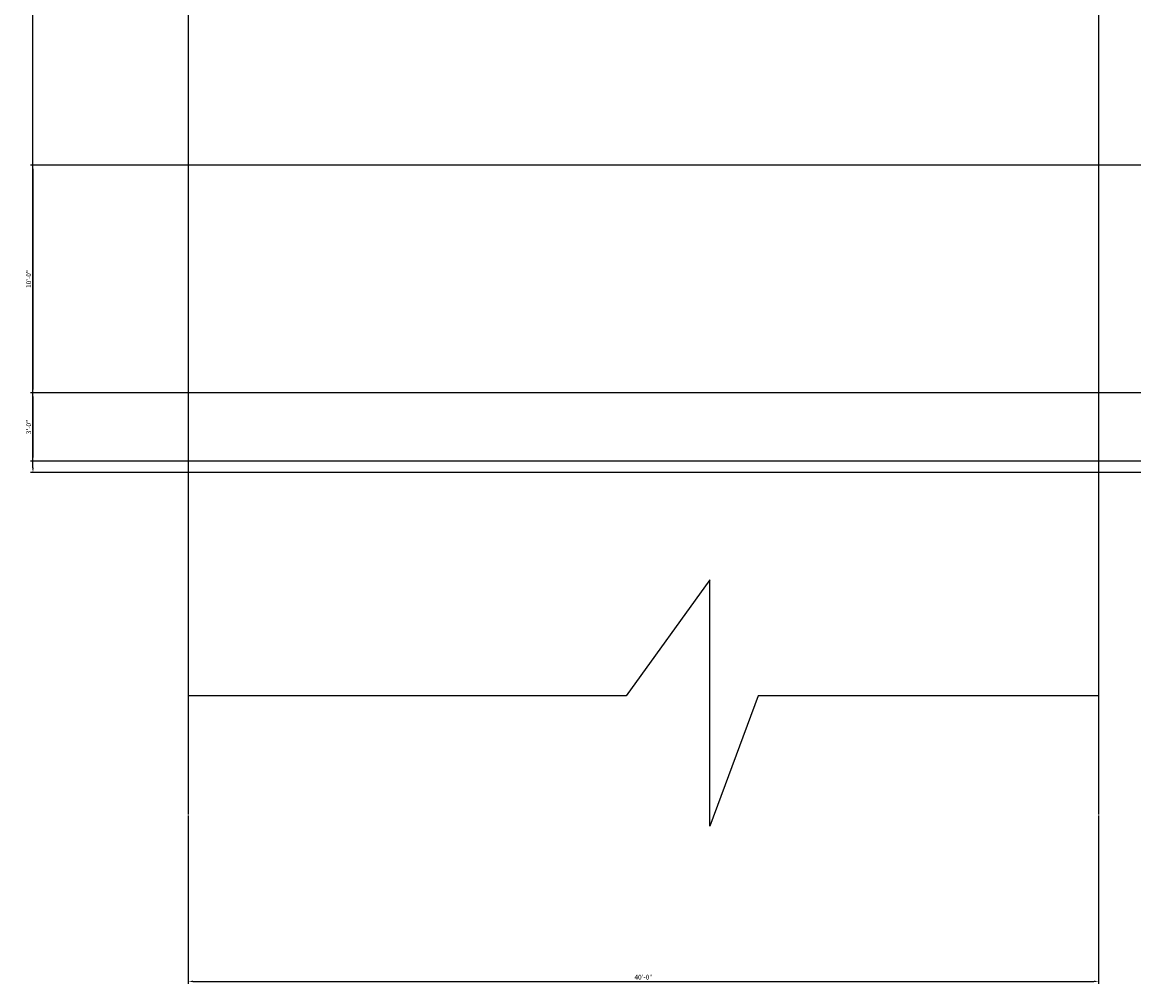
# Model space of a CAD drawing. Units: inches. Extents: x 7028582 to 7030319, y 63109697 to 63111305.
# Tile 1 of 18: x 7028582 to 7029168, y 63109697 to 63110204. Entities that reach past the tile are written whole.
import ezdxf

# ---------------------------------------------------------------- set-up
doc = ezdxf.new("R2010")
doc.units = ezdxf.units.IN
doc.layers.add('C-ANNO-DIMS', color=7, linetype='Continuous', lineweight=18)
doc.layers.add('ROAD', color=7, linetype='Continuous', lineweight=25)
doc.styles.get("Standard").update_dxf_attribs({"font": 'arial.ttf'})
doc.dimstyles.new('ISO-25', dxfattribs={"dimtxt": 2.5, "dimasz": 2.5, "dimexe": 1.25, "dimexo": 0.625, "dimtad": 1, "dimlunit": 4, "dimtxsty": 'Standard', "dimcen": 2.5, "dimadec": 0, "dimazin": 0, "dimtfac": 1, "dimtmove": 0, "dimatfit": 3, "dimfxl": 1, "dimarcsym": 0})

# ---------------------------------------------------------------- blocks, each defined once
blk = doc.blocks.new('ROAD-BREAK-40FT')
for p, q in [((275, 129.84), (230.86, 68.64)), ((275, 0), (275, 129.84)), ((16.85, 68.64), (0, 68.64)), ((230.86, 68.64), (16.85, 68.64)), ((300.42, 68.64), (275, 0)), ((480, 68.64), (300.42, 68.64))]:
    blk.add_line(p, q)
blk = doc.blocks.new('*D100')
at = {"layer": 'C-ANNO-DIMS', "color": 0, "lineweight": -2, "transparency": 16777216}
for p, q in [((7029234.08, 63111033.06), (7028586.23, 63111033.06)), ((7028587.48, 63109969.06), (7028587.48, 63111030.56)), ((7029234.08, 63109966.56), (7028586.23, 63109966.56))]:
    blk.add_line(p, q, dxfattribs=at)
at = {"layer": 'C-ANNO-DIMS', "color": 0, "lineweight": 100, "transparency": 16777216}
for points in [[(7028587.06, 63111030.56), (7028587.89, 63111030.56), (7028587.48, 63111033.06)], [(7028587.06, 63109969.06), (7028587.89, 63109969.06), (7028587.48, 63109966.56)]]:
    blk.add_solid(points, dxfattribs=at)
at = {"layer": 'Defpoints', "color": 0, "lineweight": 100, "transparency": 16777216}
for p in [(7028587.48, 63111033.06), (7029234.71, 63111033.06), (7029234.71, 63109966.56)]:
    blk.add_point(p, dxfattribs=at)
at = {"layer": 'C-ANNO-DIMS', "color": 0, "transparency": 16777216, "insert": (7028585.56, 63110499.81), "char_height": 2.5, "attachment_point": 5, "rotation": 90}
blk.add_mtext('88\'-10 1/2"', dxfattribs=at)
blk = doc.blocks.new('*D107')
at = {"layer": 'C-ANNO-DIMS', "color": 0, "lineweight": -2, "transparency": 16777216}
for p, q in [((7028669.33, 63109785.8), (7028669.33, 63109697.14)), ((7029149.33, 63109785.8), (7029149.33, 63109697.14)), ((7028671.83, 63109698.39), (7029146.83, 63109698.39))]:
    blk.add_line(p, q, dxfattribs=at)
at = {"layer": 'C-ANNO-DIMS', "color": 0, "lineweight": 100, "transparency": 16777216}
for points in [[(7028671.83, 63109698.8), (7028671.83, 63109697.97), (7028669.33, 63109698.39)], [(7029146.83, 63109698.8), (7029146.83, 63109697.97), (7029149.33, 63109698.39)]]:
    blk.add_solid(points, dxfattribs=at)
at = {"layer": 'Defpoints', "color": 0, "lineweight": 100, "transparency": 16777216}
for p in [(7028669.33, 63109786.42), (7029149.33, 63109786.42), (7029149.33, 63109698.39)]:
    blk.add_point(p, dxfattribs=at)
at = {"layer": 'C-ANNO-DIMS', "color": 0, "transparency": 16777216, "insert": (7028909.33, 63109700.29), "char_height": 2.5, "attachment_point": 5}
blk.add_mtext('40\'-0"', dxfattribs=at)
blk = doc.blocks.new('*D109')
at = {"layer": 'C-ANNO-DIMS', "color": 0, "lineweight": -2, "transparency": 16777216}
for p, q in [((7029710.58, 63110128.56), (7028586.23, 63110128.56)), ((7028587.48, 63110126.06), (7028587.48, 63110011.06)), ((7029710.58, 63110008.56), (7028586.23, 63110008.56))]:
    blk.add_line(p, q, dxfattribs=at)
at = {"layer": 'C-ANNO-DIMS', "color": 0, "lineweight": 100, "transparency": 16777216}
for points in [[(7028587.06, 63110126.06), (7028587.89, 63110126.06), (7028587.48, 63110128.56)], [(7028587.06, 63110011.06), (7028587.89, 63110011.06), (7028587.48, 63110008.56)]]:
    blk.add_solid(points, dxfattribs=at)
at = {"layer": 'Defpoints', "color": 0, "lineweight": 100, "transparency": 16777216}
for p in [(7029711.21, 63110128.56), (7028587.48, 63110008.56), (7029711.21, 63110008.56)]:
    blk.add_point(p, dxfattribs=at)
at = {"layer": 'C-ANNO-DIMS', "color": 0, "transparency": 16777216, "insert": (7028585.57, 63110068.56), "char_height": 2.5, "attachment_point": 5, "rotation": 90}
blk.add_mtext('10\'-0"', dxfattribs=at)
blk = doc.blocks.new('*D110')
at = {"layer": 'C-ANNO-DIMS', "color": 0, "lineweight": -2, "transparency": 16777216}
for p, q in [((7029747.58, 63110008.56), (7028586.23, 63110008.56)), ((7028587.48, 63110006.06), (7028587.48, 63109975.06)), ((7029747.58, 63109972.56), (7028586.23, 63109972.56))]:
    blk.add_line(p, q, dxfattribs=at)
at = {"layer": 'C-ANNO-DIMS', "color": 0, "lineweight": 100, "transparency": 16777216}
for points in [[(7028587.06, 63110006.06), (7028587.89, 63110006.06), (7028587.48, 63110008.56)], [(7028587.06, 63109975.06), (7028587.89, 63109975.06), (7028587.48, 63109972.56)]]:
    blk.add_solid(points, dxfattribs=at)
at = {"layer": 'Defpoints', "color": 0, "lineweight": 100, "transparency": 16777216}
for p in [(7029748.21, 63110008.56), (7028587.48, 63109972.56), (7029748.21, 63109972.56)]:
    blk.add_point(p, dxfattribs=at)
at = {"layer": 'C-ANNO-DIMS', "color": 0, "transparency": 16777216, "insert": (7028585.57, 63109990.56), "char_height": 2.5, "attachment_point": 5, "rotation": 90}
blk.add_mtext('3\'-0"', dxfattribs=at)

msp = doc.modelspace()

# ---------------------------------------------------------------- linework, layer by layer
at = {"layer": 'ROAD'}
for p, q in [((7028669.325, 63111208.99), (7028669.325, 63109786.421)), ((7029149.325, 63111208.99), (7029149.325, 63109786.421))]:
    msp.add_line(p, q, dxfattribs=at)

# ---------------------------------------------------------------- block references
msp.add_blockref('ROAD-BREAK-40FT', (7028669.325, 63109780.235), dxfattribs=at)

# ---------------------------------------------------------------- dimensions: what is measured, and where the dimension line sits
at = {"layer": 'C-ANNO-DIMS'}
for base, p1, p2, picture, middle in [((7028587.475, 63111033.057), (7029234.705, 63109966.557), (7029234.705, 63111033.057), '*D100', (7028585.558, 63110499.807)), ((7028587.475, 63110008.557), (7029711.205, 63110128.557), (7029711.205, 63110008.557), '*D109', (7028585.574, 63110068.557)), ((7028587.475, 63109972.557), (7029748.205, 63110008.557), (7029748.205, 63109972.557), '*D110', (7028585.573, 63109990.557))]:
    dim = msp.add_linear_dim(base=base, p1=p1, p2=p2, angle=90, dimstyle='ISO-25', override={"dimdec": 1, "dimlfac": 1, "dimrnd": 0, "dimzin": 1, "dimdsep": 46, "dimlunit": 4, "dimfrac": 2}, dxfattribs=at)
    dim.commit()
    dim.dimension.update_dxf_attribs({"geometry": picture, "text_midpoint": middle})
dim = msp.add_linear_dim(base=(7029149.325, 63109698.385), p1=(7028669.325, 63109786.421), p2=(7029149.325, 63109786.421), dimstyle='ISO-25', override={"dimdec": 1, "dimlfac": 1, "dimrnd": 0, "dimzin": 1, "dimdsep": 46, "dimlunit": 4, "dimfrac": 2}, dxfattribs=at)
dim.commit()
dim.dimension.update_dxf_attribs({"geometry": '*D107', "text_midpoint": (7028909.325, 63109700.287)})

doc.saveas('drawing.dxf')
